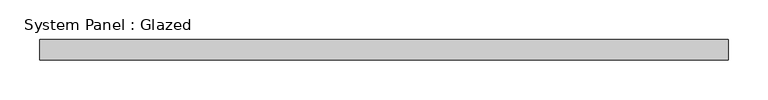
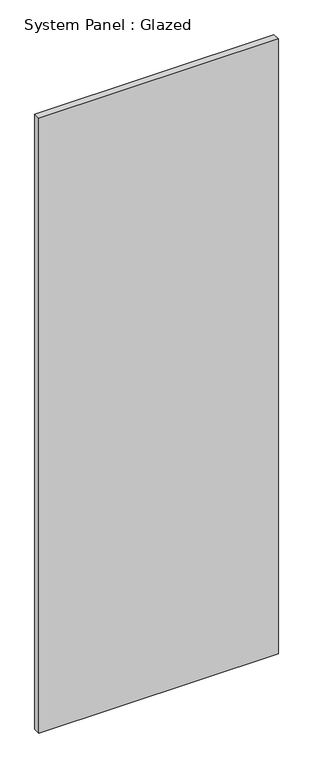
"""IFC4 building model written with IfcOpenShell, lengths in millimetres: plate geometry, System Panel : Glazed."""

from ifc_helpers import new_model, si_unit, origin, origin_with_axes, place, context, project, spatial, polyline, outline, extrude, source, transform, mapped, element, save


def system_panel_glazed_828cd182(model_context):
    return source(origin(), model_context, "Body", "SweptSolid", [
        extrude(outline(polyline([(431.8, 19.05), (-431.8, 19.05), (-431.8, 44.45), (431.8, 44.45), (431.8, 19.05)])), origin_with_axes(), (0.0, 0.0, 1.0), 2343.15),
    ])


if __name__ == "__main__":
    model = new_model("IFC4")
    model_context = context("Model", 3, world=origin())
    ifc_project = project(units=[si_unit("LENGTHUNIT", "METRE", prefix="MILLI")], contexts=[model_context])
    site = spatial("IfcSite", under=ifc_project)
    building = spatial("IfcBuilding", under=site)
    placement = place(None, origin())
    system_panel_glazed_shape = system_panel_glazed_828cd182(model_context)
    element("IfcPlate", 1, ObjectType="System Panel : Glazed", at=placement, inside=building, context=model_context, shape_type="MappedRepresentation", body=[
        mapped(system_panel_glazed_shape, transform((0.0, 0.0, 0.0), x_axis=(1.0, 0.0, 0.0), y_axis=(0.0, 1.0, 0.0), z_axis=(0.0, 0.0, 1.0))),
    ])
    save(model, "model.ifc")

# Revit data of these elements
# Type "System Panel : Glazed"
#   Construction Type Id = "GSP4R"
#   Analytic Construction = "1/8 in Pilkington single glazing"
#   Visual Light Transmittance = 0.9
#   Solar Heat Gain Coefficient = 0.86
#   Heat Transfer Coefficient (U) = 1.18115 BTU/(h·ft²·°F)
#   Define Thermal Properties by = 1
# Element 1 (IfcPlate, "System Panel : Glazed")
#   Materials on its faces: "Glass"
# Materials
#   "Glass": class "Glass", colour RGB 0 128 192, transparency 0.75, Description = "Soda Lime Glass", Cost = 0
